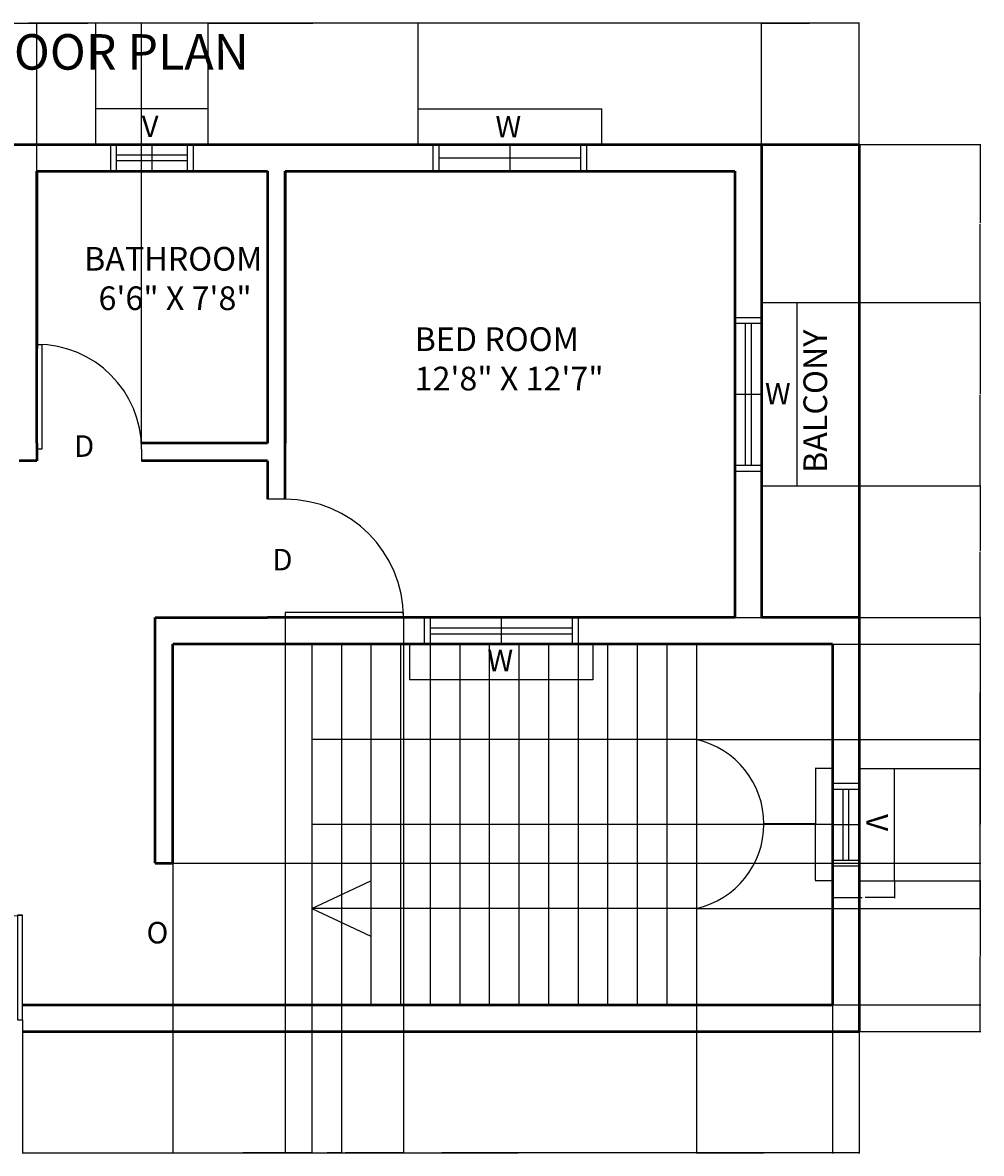
# Model space of a CAD drawing. Units: inches. Extents: x -73 to 1162, y -188 to 590.
# Tile 8 of 9: x 808 to 1132, y -187 to 195. Entities that reach past the tile are written whole.
import ezdxf

# ---------------------------------------------------------------- set-up
doc = ezdxf.new("R2010")
doc.units = ezdxf.units.IN
doc.header["$MEASUREMENT"] = 0
for name, color, linetype, lineweight in [('A-ANNO-DIMS', 2, 'Continuous', 18), ('A-ANNO-TEXT', 7, 'Continuous', 25), ('A-AREA-IDEN', 2, 'Continuous', 25), ('A-DOOR', 3, 'Continuous', 25), ('A-FLOR-STRS', 3, 'Continuous', 25), ('A-GLAZ', 4, 'Continuous', 25), ('A-WALL', 7, 'Continuous', 50)]:
    doc.layers.add(name, color=color, linetype=linetype, lineweight=lineweight)
doc.styles.get("Standard").update_dxf_attribs({"font": 'arial.ttf'})
doc.dimstyles.get("Standard").update_dxf_attribs({"dimtxt": 0.18, "dimasz": 0.18, "dimexe": 0.18, "dimexo": 0.0625, "dimgap": 0.09, "dimtad": 0, "dimtih": 1, "dimtoh": 1, "dimdec": 1, "dimzin": 0, "dimdsep": 46, "dimlunit": 4, "dimtxsty": 'Standard', "dimcen": 0.09, "dimadec": 0, "dimazin": 0, "dimtfac": 1, "dimtdec": 1, "dimtofl": 0, "dimtmove": 0, "dimatfit": 3, "dimfxl": 1, "dimtolj": 1, "dimtzin": 0, "dimarcsym": 0})

# ---------------------------------------------------------------- blocks, each defined once
blk = doc.blocks.new('*U4')
for p, q in [((0, 0), (0, -100)), ((900, 0), (900, -100))]:
    blk.add_line(p, q)
blk.add_lwpolyline([(0, 0), (0, 900), (43.75, 900), (43.75, 0)], close=True)
blk.add_arc((0, 0), 900, 0, 90)
blk = doc.blocks.new('*U7')
for p, q in [((0, 0), (0, 6)), ((40, 0), (40, 6))]:
    blk.add_line(p, q)
blk.add_lwpolyline([(0, 0), (0, -40), (1.75, -40), (1.75, 0)], close=True)
blk.add_arc((0, 0), 40, 270, 360)
blk = doc.blocks.new('WIN-W')
for p, q in [((9, 57), (9, 62)), ((9, 62), (21, 62)), ((21, 62), (21, 0)), ((0, 57), (9, 57)), ((0, 5), (9, 5)), ((9, 5), (9, 0)), ((9, 0), (21, 0))]:
    blk.add_line(p, q)
blk = doc.blocks.new('VENT-V')
for p, q in [((0, 9), (0, 21)), ((38, 21), (0, 21)), ((38, 9), (38, 21)), ((5, 9), (0, 9)), ((5, 0), (5, 9)), ((33, 0), (33, 9)), ((33, 9), (38, 9))]:
    blk.add_line(p, q)
blk = doc.blocks.new('*D32')
at = {"layer": 'A-ANNO-DIMS', "color": 0, "lineweight": -2, "transparency": 16777216}
for p, q in [((1081.24, -56.91), (1075.43, -56.91)), ((1075.61, -57.09), (1075.61, -75.72)), ((1075.61, -94.73), (1075.61, -76.09)), ((1081.24, -94.91), (1075.43, -94.91))]:
    blk.add_line(p, q, dxfattribs=at)
at = {"layer": 'A-ANNO-DIMS', "color": 0, "transparency": 16777216}
for points in [[(1075.58, -57.09), (1075.64, -57.09), (1075.61, -56.91)], [(1075.58, -94.73), (1075.64, -94.73), (1075.61, -94.91)]]:
    blk.add_solid(points, dxfattribs=at)
at = {"layer": 'Defpoints', "color": 0, "transparency": 16777216}
for p in [(1081.31, -56.91), (1075.61, -94.91), (1081.31, -94.91)]:
    blk.add_point(p, dxfattribs=at)
at = {"layer": 'A-ANNO-DIMS', "color": 0, "transparency": 16777216, "insert": (1075.61, -75.91), "char_height": 0.18, "attachment_point": 5}
blk.add_mtext('\\A1;VENTILATOR V 38 TYP.', dxfattribs=at)
blk = doc.blocks.new('*D33')
at = {"layer": 'A-ANNO-DIMS', "color": 0, "lineweight": -2, "transparency": 16777216}
for p, q in [((1081.31, -94.97), (1081.31, -100.79)), ((1102.31, -94.97), (1102.31, -100.79)), ((1081.49, -100.61), (1091.28, -100.61)), ((1102.13, -100.61), (1092.34, -100.61))]:
    blk.add_line(p, q, dxfattribs=at)
at = {"layer": 'A-ANNO-DIMS', "color": 0, "transparency": 16777216}
for points in [[(1081.49, -100.58), (1081.49, -100.64), (1081.31, -100.61)], [(1102.13, -100.58), (1102.13, -100.64), (1102.31, -100.61)]]:
    blk.add_solid(points, dxfattribs=at)
at = {"layer": 'Defpoints', "color": 0, "transparency": 16777216}
for p in [(1081.31, -94.91), (1102.31, -94.91), (1102.31, -100.61)]:
    blk.add_point(p, dxfattribs=at)
at = {"layer": 'A-ANNO-DIMS', "color": 0, "transparency": 16777216, "insert": (1091.81, -100.61), "char_height": 0.18, "attachment_point": 5}
blk.add_mtext('\\A1;21 TYP.', dxfattribs=at)
blk = doc.blocks.new('*D100')
at = {"layer": 'A-ANNO-DIMS', "color": 0, "lineweight": -2, "transparency": 16777216}
for p, q in [((557.31, 154.15), (557.31, 195.27)), ((557.49, 195.09), (823.52, 195.09)), ((1090.13, 195.09), (824.1, 195.09)), ((1090.31, 154.15), (1090.31, 195.27))]:
    blk.add_line(p, q, dxfattribs=at)
at = {"layer": 'A-ANNO-DIMS', "color": 0, "transparency": 16777216}
for points in [[(557.49, 195.12), (557.49, 195.06), (557.31, 195.09)], [(1090.13, 195.12), (1090.13, 195.06), (1090.31, 195.09)]]:
    blk.add_solid(points, dxfattribs=at)
at = {"layer": 'Defpoints', "color": 0, "transparency": 16777216}
for p in [(1090.31, 195.09), (557.31, 154.09), (1090.31, 154.09)]:
    blk.add_point(p, dxfattribs=at)
at = {"layer": 'A-ANNO-DIMS', "color": 0, "transparency": 16777216, "insert": (823.81, 195.09), "char_height": 0.18, "attachment_point": 5}
blk.add_mtext('\\A1;533', dxfattribs=at)
blk = doc.blocks.new('*D102')
at = {"layer": 'A-ANNO-DIMS', "color": 0, "lineweight": -2, "transparency": 16777216}
for p, q in [((786.31, 166.15), (786.31, 195.27)), ((786.49, 195.09), (809.08, 195.09)), ((832.13, 195.09), (809.53, 195.09)), ((832.31, 166.15), (832.31, 195.27))]:
    blk.add_line(p, q, dxfattribs=at)
at = {"layer": 'A-ANNO-DIMS', "color": 0, "transparency": 16777216}
for points in [[(786.49, 195.12), (786.49, 195.06), (786.31, 195.09)], [(832.13, 195.12), (832.13, 195.06), (832.31, 195.09)]]:
    blk.add_solid(points, dxfattribs=at)
at = {"layer": 'Defpoints', "color": 0, "transparency": 16777216}
for p in [(832.31, 195.09), (786.31, 166.09), (832.31, 166.09)]:
    blk.add_point(p, dxfattribs=at)
at = {"layer": 'A-ANNO-DIMS', "color": 0, "transparency": 16777216, "insert": (809.31, 195.09), "char_height": 0.18, "attachment_point": 5}
blk.add_mtext('\\A1;46', dxfattribs=at)
blk = doc.blocks.new('*D103')
at = {"layer": 'A-ANNO-DIMS', "color": 0, "lineweight": -2, "transparency": 16777216}
for p, q in [((870.31, 166.15), (870.31, 195.27)), ((870.49, 195.09), (905.61, 195.09)), ((941.13, 195.09), (906.01, 195.09)), ((941.31, 166.15), (941.31, 195.27))]:
    blk.add_line(p, q, dxfattribs=at)
at = {"layer": 'A-ANNO-DIMS', "color": 0, "transparency": 16777216}
for points in [[(870.49, 195.12), (870.49, 195.06), (870.31, 195.09)], [(941.13, 195.12), (941.13, 195.06), (941.31, 195.09)]]:
    blk.add_solid(points, dxfattribs=at)
at = {"layer": 'Defpoints', "color": 0, "transparency": 16777216}
for p in [(941.31, 195.09), (870.31, 166.09), (941.31, 166.09)]:
    blk.add_point(p, dxfattribs=at)
at = {"layer": 'A-ANNO-DIMS', "color": 0, "transparency": 16777216, "insert": (905.81, 195.09), "char_height": 0.18, "attachment_point": 5}
blk.add_mtext('\\A1;71', dxfattribs=at)
blk = doc.blocks.new('*D111')
at = {"layer": 'A-ANNO-DIMS', "color": 0, "lineweight": -2, "transparency": 16777216}
for p, q in [((807.52, -145.97), (807.52, -187.09)), ((1090.31, -145.97), (1090.31, -187.09)), ((807.7, -186.91), (948.52, -186.91)), ((1090.13, -186.91), (949.31, -186.91))]:
    blk.add_line(p, q, dxfattribs=at)
at = {"layer": 'A-ANNO-DIMS', "color": 0, "transparency": 16777216}
for points in [[(807.7, -186.88), (807.7, -186.94), (807.52, -186.91)], [(1090.13, -186.88), (1090.13, -186.94), (1090.31, -186.91)]]:
    blk.add_solid(points, dxfattribs=at)
at = {"layer": 'Defpoints', "color": 0, "transparency": 16777216}
for p in [(807.52, -145.91), (1090.31, -145.91), (1090.31, -186.91)]:
    blk.add_point(p, dxfattribs=at)
at = {"layer": 'A-ANNO-DIMS', "color": 0, "transparency": 16777216, "insert": (948.91, -186.91), "char_height": 0.18, "attachment_point": 5}
blk.add_mtext('\\A1;282.8', dxfattribs=at)
blk = doc.blocks.new('*D112')
at = {"layer": 'A-ANNO-DIMS', "color": 0, "lineweight": -2, "transparency": 16777216}
for p, q in [((1090.37, 154.09), (1131.49, 154.09)), ((1131.31, 153.91), (1131.31, 127.52)), ((1131.31, 100.77), (1131.31, 127.16)), ((1069.37, 100.59), (1131.49, 100.59))]:
    blk.add_line(p, q, dxfattribs=at)
at = {"layer": 'A-ANNO-DIMS', "color": 0, "transparency": 16777216}
for points in [[(1131.28, 153.91), (1131.34, 153.91), (1131.31, 154.09)], [(1131.28, 100.77), (1131.34, 100.77), (1131.31, 100.59)]]:
    blk.add_solid(points, dxfattribs=at)
at = {"layer": 'Defpoints', "color": 0, "transparency": 16777216}
for p in [(1090.31, 154.09), (1069.31, 100.59), (1131.31, 100.59)]:
    blk.add_point(p, dxfattribs=at)
at = {"layer": 'A-ANNO-DIMS', "color": 0, "transparency": 16777216, "insert": (1131.31, 127.34), "char_height": 0.18, "attachment_point": 5}
blk.add_mtext('\\A1;53.5', dxfattribs=at)
blk = doc.blocks.new('*D113')
at = {"layer": 'A-ANNO-DIMS', "color": 0, "lineweight": -2, "transparency": 16777216}
for p, q in [((1069.37, 100.59), (1131.49, 100.59)), ((1131.31, 100.41), (1131.31, 69.77)), ((1131.31, 38.77), (1131.31, 69.41)), ((1069.37, 38.59), (1131.49, 38.59))]:
    blk.add_line(p, q, dxfattribs=at)
at = {"layer": 'A-ANNO-DIMS', "color": 0, "transparency": 16777216}
for points in [[(1131.28, 100.41), (1131.34, 100.41), (1131.31, 100.59)], [(1131.28, 38.77), (1131.34, 38.77), (1131.31, 38.59)]]:
    blk.add_solid(points, dxfattribs=at)
at = {"layer": 'Defpoints', "color": 0, "transparency": 16777216}
for p in [(1069.31, 100.59), (1069.31, 38.59), (1131.31, 38.59)]:
    blk.add_point(p, dxfattribs=at)
at = {"layer": 'A-ANNO-DIMS', "color": 0, "transparency": 16777216, "insert": (1131.31, 69.59), "char_height": 0.18, "attachment_point": 5}
blk.add_mtext('\\A1;62', dxfattribs=at)
blk = doc.blocks.new('*D114')
at = {"layer": 'A-ANNO-DIMS', "color": 0, "lineweight": -2, "transparency": 16777216}
for p, q in [((1069.37, 38.59), (1131.49, 38.59)), ((1131.31, 38.41), (1131.31, 16.52)), ((1131.31, -5.73), (1131.31, 16.16)), ((1090.37, -5.91), (1131.49, -5.91))]:
    blk.add_line(p, q, dxfattribs=at)
at = {"layer": 'A-ANNO-DIMS', "color": 0, "transparency": 16777216}
for points in [[(1131.28, 38.41), (1131.34, 38.41), (1131.31, 38.59)], [(1131.28, -5.73), (1131.34, -5.73), (1131.31, -5.91)]]:
    blk.add_solid(points, dxfattribs=at)
at = {"layer": 'Defpoints', "color": 0, "transparency": 16777216}
for p in [(1069.31, 38.59), (1090.31, -5.91), (1131.31, -5.91)]:
    blk.add_point(p, dxfattribs=at)
at = {"layer": 'A-ANNO-DIMS', "color": 0, "transparency": 16777216, "insert": (1131.31, 16.34), "char_height": 0.18, "attachment_point": 5}
blk.add_mtext('\\A1;44.5', dxfattribs=at)
blk = doc.blocks.new('*D115')
at = {"layer": 'A-ANNO-DIMS', "color": 0, "lineweight": -2, "transparency": 16777216}
for p, q in [((1090.37, -5.91), (1131.49, -5.91)), ((1131.31, -6.09), (1131.31, -31.23)), ((1131.31, -56.73), (1131.31, -31.59)), ((1090.37, -56.91), (1131.49, -56.91))]:
    blk.add_line(p, q, dxfattribs=at)
at = {"layer": 'A-ANNO-DIMS', "color": 0, "transparency": 16777216}
for points in [[(1131.28, -6.09), (1131.34, -6.09), (1131.31, -5.91)], [(1131.28, -56.73), (1131.34, -56.73), (1131.31, -56.91)]]:
    blk.add_solid(points, dxfattribs=at)
at = {"layer": 'Defpoints', "color": 0, "transparency": 16777216}
for p in [(1090.31, -5.91), (1090.31, -56.91), (1131.31, -56.91)]:
    blk.add_point(p, dxfattribs=at)
at = {"layer": 'A-ANNO-DIMS', "color": 0, "transparency": 16777216, "insert": (1131.31, -31.41), "char_height": 0.18, "attachment_point": 5}
blk.add_mtext('\\A1;51', dxfattribs=at)
blk = doc.blocks.new('*D116')
at = {"layer": 'A-ANNO-DIMS', "color": 0, "lineweight": -2, "transparency": 16777216}
for p, q in [((1090.37, -94.91), (1131.49, -94.91)), ((1131.31, -95.09), (1131.31, -120.23)), ((1131.31, -145.73), (1131.31, -120.59)), ((1090.37, -145.91), (1131.49, -145.91))]:
    blk.add_line(p, q, dxfattribs=at)
at = {"layer": 'A-ANNO-DIMS', "color": 0, "transparency": 16777216}
for points in [[(1131.28, -95.09), (1131.34, -95.09), (1131.31, -94.91)], [(1131.28, -145.73), (1131.34, -145.73), (1131.31, -145.91)]]:
    blk.add_solid(points, dxfattribs=at)
at = {"layer": 'Defpoints', "color": 0, "transparency": 16777216}
for p in [(1090.31, -94.91), (1090.31, -145.91), (1131.31, -145.91)]:
    blk.add_point(p, dxfattribs=at)
at = {"layer": 'A-ANNO-DIMS', "color": 0, "transparency": 16777216, "insert": (1131.31, -120.41), "char_height": 0.18, "attachment_point": 5}
blk.add_mtext('\\A1;51', dxfattribs=at)
blk = doc.blocks.new('*D118')
at = {"layer": 'A-ANNO-DIMS', "color": 0, "lineweight": -2, "transparency": 16777216}
for p, q in [((812.31, 53.15), (812.31, 195.27)), ((812.49, 195.09), (829.6, 195.09)), ((847.5, 195.09), (830.39, 195.09)), ((847.68, 53.15), (847.68, 195.27))]:
    blk.add_line(p, q, dxfattribs=at)
at = {"layer": 'A-ANNO-DIMS', "color": 0, "transparency": 16777216}
for points in [[(812.49, 195.12), (812.49, 195.06), (812.31, 195.09)], [(847.5, 195.12), (847.5, 195.06), (847.68, 195.09)]]:
    blk.add_solid(points, dxfattribs=at)
at = {"layer": 'Defpoints', "color": 0, "transparency": 16777216}
for p in [(847.68, 195.09), (812.31, 53.09), (847.68, 53.09)]:
    blk.add_point(p, dxfattribs=at)
at = {"layer": 'A-ANNO-DIMS', "color": 0, "transparency": 16777216, "insert": (829.99, 195.09), "char_height": 0.18, "attachment_point": 5}
blk.add_mtext('\\A1;35.37', dxfattribs=at)
blk = doc.blocks.new('*D119')
at = {"layer": 'A-ANNO-DIMS', "color": 0, "lineweight": -2, "transparency": 16777216}
for p, q in [((858.31, -14.97), (858.31, -187.09)), ((905.31, -14.97), (905.31, -187.09)), ((858.49, -186.91), (881.58, -186.91)), ((905.13, -186.91), (882.03, -186.91))]:
    blk.add_line(p, q, dxfattribs=at)
at = {"layer": 'A-ANNO-DIMS', "color": 0, "transparency": 16777216}
for points in [[(858.49, -186.88), (858.49, -186.94), (858.31, -186.91)], [(905.13, -186.88), (905.13, -186.94), (905.31, -186.91)]]:
    blk.add_solid(points, dxfattribs=at)
at = {"layer": 'Defpoints', "color": 0, "transparency": 16777216}
for p in [(858.31, -14.91), (905.31, -14.91), (905.31, -186.91)]:
    blk.add_point(p, dxfattribs=at)
at = {"layer": 'A-ANNO-DIMS', "color": 0, "transparency": 16777216, "insert": (881.81, -186.91), "char_height": 0.18, "attachment_point": 5}
blk.add_mtext('\\A1;47', dxfattribs=at)
blk = doc.blocks.new('*D120')
at = {"layer": 'A-ANNO-DIMS', "color": 0, "lineweight": -2, "transparency": 16777216}
for p, q in [((905.31, -14.97), (905.31, -187.09)), ((915.31, -14.97), (915.31, -187.09)), ((905.49, -186.91), (910.1, -186.91)), ((915.13, -186.91), (910.52, -186.91))]:
    blk.add_line(p, q, dxfattribs=at)
at = {"layer": 'A-ANNO-DIMS', "color": 0, "transparency": 16777216}
for points in [[(905.49, -186.88), (905.49, -186.94), (905.31, -186.91)], [(915.13, -186.88), (915.13, -186.94), (915.31, -186.91)]]:
    blk.add_solid(points, dxfattribs=at)
at = {"layer": 'Defpoints', "color": 0, "transparency": 16777216}
for p in [(905.31, -14.91), (915.31, -14.91), (915.31, -186.91)]:
    blk.add_point(p, dxfattribs=at)
at = {"layer": 'A-ANNO-DIMS', "color": 0, "transparency": 16777216, "insert": (910.31, -186.91), "char_height": 0.18, "attachment_point": 5}
blk.add_mtext('\\A1;10', dxfattribs=at)
blk = doc.blocks.new('*D121')
at = {"layer": 'A-ANNO-DIMS', "color": 0, "lineweight": -2, "transparency": 16777216}
for p, q in [((915.31, -14.97), (915.31, -187.09)), ((1035.31, -14.97), (1035.31, -187.09)), ((915.49, -186.91), (975.03, -186.91)), ((1035.13, -186.91), (975.59, -186.91))]:
    blk.add_line(p, q, dxfattribs=at)
at = {"layer": 'A-ANNO-DIMS', "color": 0, "transparency": 16777216}
for points in [[(915.49, -186.88), (915.49, -186.94), (915.31, -186.91)], [(1035.13, -186.88), (1035.13, -186.94), (1035.31, -186.91)]]:
    blk.add_solid(points, dxfattribs=at)
at = {"layer": 'Defpoints', "color": 0, "transparency": 16777216}
for p in [(915.31, -14.91), (1035.31, -14.91), (1035.31, -186.91)]:
    blk.add_point(p, dxfattribs=at)
at = {"layer": 'A-ANNO-DIMS', "color": 0, "transparency": 16777216, "insert": (975.31, -186.91), "char_height": 0.18, "attachment_point": 5}
blk.add_mtext('\\A1;120', dxfattribs=at)
blk = doc.blocks.new('*D122')
at = {"layer": 'A-ANNO-DIMS', "color": 0, "lineweight": -2, "transparency": 16777216}
for p, q in [((1035.31, -14.97), (1035.31, -187.09)), ((1081.31, -14.97), (1081.31, -187.09)), ((1035.49, -186.91), (1058.08, -186.91)), ((1081.13, -186.91), (1058.53, -186.91))]:
    blk.add_line(p, q, dxfattribs=at)
at = {"layer": 'A-ANNO-DIMS', "color": 0, "transparency": 16777216}
for points in [[(1035.49, -186.88), (1035.49, -186.94), (1035.31, -186.91)], [(1081.13, -186.88), (1081.13, -186.94), (1081.31, -186.91)]]:
    blk.add_solid(points, dxfattribs=at)
at = {"layer": 'Defpoints', "color": 0, "transparency": 16777216}
for p in [(1035.31, -14.91), (1081.31, -14.91), (1081.31, -186.91)]:
    blk.add_point(p, dxfattribs=at)
at = {"layer": 'A-ANNO-DIMS', "color": 0, "transparency": 16777216, "insert": (1058.31, -186.91), "char_height": 0.18, "attachment_point": 5}
blk.add_mtext('\\A1;46', dxfattribs=at)
blk = doc.blocks.new('*D123')
at = {"layer": 'A-ANNO-DIMS', "color": 0, "lineweight": -2, "transparency": 16777216}
for p, q in [((852.37, -5.91), (1131.49, -5.91)), ((1131.31, -6.09), (1131.31, -47.23)), ((1131.31, -88.73), (1131.31, -47.59)), ((852.37, -88.91), (1131.49, -88.91))]:
    blk.add_line(p, q, dxfattribs=at)
at = {"layer": 'A-ANNO-DIMS', "color": 0, "transparency": 16777216}
for points in [[(1131.28, -6.09), (1131.34, -6.09), (1131.31, -5.91)], [(1131.28, -88.73), (1131.34, -88.73), (1131.31, -88.91)]]:
    blk.add_solid(points, dxfattribs=at)
at = {"layer": 'Defpoints', "color": 0, "transparency": 16777216}
for p in [(852.31, -5.91), (1131.31, -5.91), (852.31, -88.91)]:
    blk.add_point(p, dxfattribs=at)
at = {"layer": 'A-ANNO-DIMS', "color": 0, "transparency": 16777216, "insert": (1131.31, -47.41), "char_height": 0.18, "attachment_point": 5}
blk.add_mtext('\\A1;83', dxfattribs=at)
blk = doc.blocks.new('*D124')
at = {"layer": 'A-ANNO-DIMS', "color": 0, "lineweight": -2, "transparency": 16777216}
for p, q in [((1035.37, -14.91), (1131.49, -14.91)), ((1131.31, -15.09), (1131.31, -30.86)), ((1131.31, -46.99), (1131.31, -31.22)), ((1035.37, -47.17), (1131.49, -47.17))]:
    blk.add_line(p, q, dxfattribs=at)
at = {"layer": 'A-ANNO-DIMS', "color": 0, "transparency": 16777216}
for points in [[(1131.28, -15.09), (1131.34, -15.09), (1131.31, -14.91)], [(1131.28, -46.99), (1131.34, -46.99), (1131.31, -47.17)]]:
    blk.add_solid(points, dxfattribs=at)
at = {"layer": 'Defpoints', "color": 0, "transparency": 16777216}
for p in [(1035.31, -14.91), (1035.31, -47.17), (1131.31, -47.17)]:
    blk.add_point(p, dxfattribs=at)
at = {"layer": 'A-ANNO-DIMS', "color": 0, "transparency": 16777216, "insert": (1131.31, -31.04), "char_height": 0.18, "attachment_point": 5}
blk.add_mtext('\\A1;32.264', dxfattribs=at)
blk = doc.blocks.new('*D125')
at = {"layer": 'A-ANNO-DIMS', "color": 0, "lineweight": -2, "transparency": 16777216}
for p, q in [((1035.37, -47.17), (1131.49, -47.17)), ((1131.31, -47.35), (1131.31, -75.54)), ((1131.31, -104.09), (1131.31, -75.9)), ((1035.37, -104.27), (1131.49, -104.27))]:
    blk.add_line(p, q, dxfattribs=at)
at = {"layer": 'A-ANNO-DIMS', "color": 0, "transparency": 16777216}
for points in [[(1131.28, -47.35), (1131.34, -47.35), (1131.31, -47.17)], [(1131.28, -104.09), (1131.34, -104.09), (1131.31, -104.27)]]:
    blk.add_solid(points, dxfattribs=at)
at = {"layer": 'Defpoints', "color": 0, "transparency": 16777216}
for p in [(1035.31, -47.17), (1035.31, -104.27), (1131.31, -104.27)]:
    blk.add_point(p, dxfattribs=at)
at = {"layer": 'A-ANNO-DIMS', "color": 0, "transparency": 16777216, "insert": (1131.31, -75.72), "char_height": 0.18, "attachment_point": 5}
blk.add_mtext('\\A1;57.1', dxfattribs=at)
blk = doc.blocks.new('*D126')
at = {"layer": 'A-ANNO-DIMS', "color": 0, "lineweight": -2, "transparency": 16777216}
for p, q in [((1035.37, -104.27), (1131.49, -104.27)), ((1131.31, -104.45), (1131.31, -120.41)), ((1131.31, -136.73), (1131.31, -120.77)), ((1035.37, -136.91), (1131.49, -136.91))]:
    blk.add_line(p, q, dxfattribs=at)
at = {"layer": 'A-ANNO-DIMS', "color": 0, "transparency": 16777216}
for points in [[(1131.28, -104.45), (1131.34, -104.45), (1131.31, -104.27)], [(1131.28, -136.73), (1131.34, -136.73), (1131.31, -136.91)]]:
    blk.add_solid(points, dxfattribs=at)
at = {"layer": 'Defpoints', "color": 0, "transparency": 16777216}
for p in [(1035.31, -104.27), (1035.31, -136.91), (1131.31, -136.91)]:
    blk.add_point(p, dxfattribs=at)
at = {"layer": 'A-ANNO-DIMS', "color": 0, "transparency": 16777216, "insert": (1131.31, -120.59), "char_height": 0.18, "attachment_point": 5}
blk.add_mtext('\\A1;32.64', dxfattribs=at)
blk = doc.blocks.new('*D127')
at = {"layer": 'A-ANNO-DIMS', "color": 0, "lineweight": -2, "transparency": 16777216}
for p, q in [((896.31, -5.97), (896.31, -187.09)), ((936.31, -5.97), (936.31, -187.09)), ((896.49, -186.91), (916.08, -186.91)), ((936.13, -186.91), (916.53, -186.91))]:
    blk.add_line(p, q, dxfattribs=at)
at = {"layer": 'A-ANNO-DIMS', "color": 0, "transparency": 16777216}
for points in [[(896.49, -186.88), (896.49, -186.94), (896.31, -186.91)], [(936.13, -186.88), (936.13, -186.94), (936.31, -186.91)]]:
    blk.add_solid(points, dxfattribs=at)
at = {"layer": 'Defpoints', "color": 0, "transparency": 16777216}
for p in [(896.31, -5.91), (936.31, -5.91), (936.31, -186.91)]:
    blk.add_point(p, dxfattribs=at)
at = {"layer": 'A-ANNO-DIMS', "color": 0, "transparency": 16777216, "insert": (916.31, -186.91), "char_height": 0.18, "attachment_point": 5}
blk.add_mtext('\\A1;40', dxfattribs=at)
blk = doc.blocks.new('*D128')
at = {"layer": 'A-ANNO-DIMS', "color": 0, "lineweight": -2, "transparency": 16777216}
for p, q in [((1057.31, -5.85), (1057.31, 195.27)), ((1057.49, 195.09), (1073.59, 195.09)), ((1090.13, 195.09), (1074.03, 195.09)), ((1090.31, -5.85), (1090.31, 195.27))]:
    blk.add_line(p, q, dxfattribs=at)
at = {"layer": 'A-ANNO-DIMS', "color": 0, "transparency": 16777216}
for points in [[(1057.49, 195.12), (1057.49, 195.06), (1057.31, 195.09)], [(1090.13, 195.12), (1090.13, 195.06), (1090.31, 195.09)]]:
    blk.add_solid(points, dxfattribs=at)
at = {"layer": 'Defpoints', "color": 0, "transparency": 16777216}
for p in [(1090.31, 195.09), (1057.31, -5.91), (1090.31, -5.91)]:
    blk.add_point(p, dxfattribs=at)
at = {"layer": 'A-ANNO-DIMS', "color": 0, "transparency": 16777216, "insert": (1073.81, 195.09), "char_height": 0.18, "attachment_point": 5}
blk.add_mtext('\\A1;33', dxfattribs=at)
blk = doc.blocks.new('*D162')
at = {"layer": 'A-ANNO-DIMS', "color": 0, "lineweight": -2, "transparency": 16777216}
for p, q in [((1028.8, -75.72), (1028.98, -75.72)), ((1028.89, -75.81), (1028.89, -75.63)), ((1075.7, -75.69), (1058.33, -75.7))]:
    blk.add_line(p, q, dxfattribs=at)
at = {"layer": 'A-ANNO-DIMS', "color": 0, "transparency": 16777216}
blk.add_solid([(1058.33, -75.67), (1058.33, -75.73), (1058.15, -75.7)], dxfattribs=at)
at = {"layer": 'Defpoints', "color": 0, "transparency": 16777216}
for p in [(1028.89, -75.72), (1058.15, -75.7)]:
    blk.add_point(p, dxfattribs=at)
at = {"layer": 'A-ANNO-DIMS', "color": 0, "transparency": 16777216, "insert": (1076.18, -75.69), "char_height": 0.18, "attachment_point": 5}
blk.add_mtext('\\A1;R29.26', dxfattribs=at)

msp = doc.modelspace()

# ---------------------------------------------------------------- linework, layer by layer
at = {"layer": 'A-FLOR-STRS'}
for p, q in [((905.307, -14.9077), (905.307, -136.9077)), ((915.307, -14.9077), (915.307, -136.9077)), ((925.307, -14.9077), (925.307, -136.9077)), ((935.307, -14.9077), (935.307, -136.9077)), ((945.307, -14.9077), (945.307, -136.9077)), ((955.307, -14.9077), (955.307, -136.9077)), ((965.307, -14.9077), (965.307, -136.9077)), ((975.307, -14.9077), (975.307, -136.9077)), ((985.307, -14.9077), (985.307, -136.9077)), ((995.307, -14.9077), (995.307, -136.9077)), ((1005.307, -14.9077), (1005.307, -136.9077)), ((1015.307, -14.9077), (1015.307, -136.9077)), ((1025.307, -14.9077), (1025.307, -136.9077)), ((1035.307, -14.9077), (1035.307, -136.9077)), ((1035.307, -47.1714), (905.307, -47.1714)), ((1081.307, -75.9077), (905.307, -75.9077)), ((905.307, -104.2668), (925.307, -94.9497)), ((1035.307, -104.2668), (905.307, -104.2668)), ((905.307, -104.2668), (925.307, -113.5839))]:
    msp.add_line(p, q, dxfattribs=at)
msp.add_arc((1028.8864, -75.7191), 29.2608, 282.675347, 77.324653, dxfattribs=at)
at = {"layer": 'A-GLAZ'}
for p, q in [((839.307, 145.0923), (839.307, 154.0923)), ((851.307, 145.0923), (851.307, 154.0923)), ((863.307, 145.0923), (863.307, 154.0923)), ((948.307, 145.0923), (948.307, 154.0923)), ((972.307, 145.0923), (972.307, 154.0923)), ((996.307, 145.0923), (996.307, 154.0923)), ((839.307, 150.5923), (863.307, 150.5923)), ((948.307, 149.5923), (996.307, 149.5923)), ((839.307, 148.5923), (863.307, 148.5923)), ((1048.307, 93.5923), (1057.307, 93.5923)), ((1051.807, 93.5923), (1051.807, 45.5923)), ((1053.807, 93.5923), (1053.807, 45.5923)), ((1048.307, 69.5923), (1057.307, 69.5923)), ((1048.307, 45.5923), (1057.307, 45.5923)), ((943.307, -5.9077), (943.307, -14.9077)), ((945.307, -5.9077), (945.307, -14.9077)), ((969.307, -5.9077), (969.307, -14.9077)), ((993.307, -5.9077), (993.307, -14.9077)), ((995.307, -5.9077), (995.307, -14.9077)), ((945.307, -9.4077), (993.307, -9.4077)), ((945.307, -11.4077), (993.307, -11.4077)), ((943.307, -14.9077), (938.307, -14.9077)), ((938.307, -14.9077), (938.307, -26.9077)), ((995.307, -14.9077), (1000.307, -14.9077)), ((1000.307, -14.9077), (1000.307, -26.9077)), ((1000.307, -26.9077), (938.307, -26.9077)), ((1081.307, -63.9077), (1090.307, -63.9077)), ((1084.807, -63.9077), (1084.807, -87.9077)), ((1086.807, -63.9077), (1086.807, -87.9077)), ((1081.307, -75.9077), (1090.307, -75.9077)), ((1081.307, -87.9077), (1090.307, -87.9077))]:
    msp.add_line(p, q, dxfattribs=at)
at = {"layer": 'A-WALL'}
for p, q in [((728.307, 154.0923), (812.307, 154.0923)), ((812.307, 154.0923), (896.307, 154.0923)), ((896.307, 154.0923), (1090.307, 154.0923)), ((1057.307, 154.0923), (1057.307, -5.9077)), ((1090.307, 154.0923), (1090.307, -5.9077)), ((812.307, 145.0923), (812.307, 85.0923)), ((812.307, 145.0923), (890.307, 145.0923)), ((812.307, 53.0923), (812.307, 145.0923)), ((890.307, 145.0923), (890.307, 53.0923)), ((896.307, 145.0923), (896.307, 53.0923)), ((896.307, 145.0923), (1048.307, 145.0923)), ((896.307, 34.0923), (896.307, 145.0923)), ((1048.307, 145.0923), (1048.307, -5.9077)), ((812.307, 53.0923), (812.307, 47.0923)), ((890.307, 53.0923), (847.68, 53.0923)), ((812.307, 47.0923), (806.307, 47.0923)), ((890.307, 47.0923), (847.7401, 47.0923)), ((890.307, 47.0923), (890.307, 34.0923)), ((852.307, -88.9077), (852.307, -5.9077)), ((852.307, -5.9077), (890.307, -5.9077)), ((1048.307, -5.9077), (890.307, -5.9077)), ((1090.307, -5.9077), (1057.307, -5.9077)), ((1090.307, -5.9077), (1090.307, -145.9077)), ((1081.307, -14.9077), (858.307, -14.9077)), ((858.307, -88.9077), (858.307, -14.9077)), ((1081.307, -14.9077), (1081.307, -136.9077)), ((852.307, -88.9077), (858.307, -88.9077)), ((807.5207, -136.9077), (852.307, -136.9077)), ((852.307, -136.9077), (1081.307, -136.9077)), ((807.5207, -145.9077), (1090.307, -145.9077))]:
    msp.add_line(p, q, dxfattribs=at)

# ---------------------------------------------------------------- block references
at = {"layer": 'A-DOOR', "yscale": 0.0393700787401575, "zscale": 0.0393700787401575}
for p, xscale in [((812.307, 51.0293), 0.0393700787401575), ((807.5207, -141.9707), -0.0393700787401575)]:
    msp.add_blockref('*U4', p, dxfattribs=dict(at, xscale=xscale))
at = {"layer": 'A-DOOR', "rotation": 90}
msp.add_blockref('*U7', (896.307, -5.9077), dxfattribs=at)
at = {"layer": 'A-GLAZ'}
for name, p in [('VENT-V', (832.307, 145.0919)), ('WIN-W', (1048.307, 38.5919))]:
    msp.add_blockref(name, p, dxfattribs=at)
for name, p, rotation in [('WIN-W', (1003.3075, 145.0923), 90.00000000000021), ('VENT-V', (1081.3066, -56.9077), 269.999999999999)]:
    msp.add_blockref(name, p, dxfattribs=dict(at, rotation=rotation))

# ---------------------------------------------------------------- texts
at = {"layer": 'A-ANNO-TEXT'}
for s, p in [('V', (847.7724, 156.5575)), ('W', (967.3667, 156.4655)), ('W', (1058.4992, 66.1733)), ('D', (824.9009, 48.444)), ('D', (891.9441, 10.0239)), ('W', (964.6447, -24.0471)), ('O', (849.4199, -116.0969))]:
    msp.add_text(s, height=7.2829, dxfattribs=at).set_placement(p)
msp.add_text('V', height=7.2829, rotation=270, dxfattribs=at).set_placement((1092.7722, -72.3731))
at = {"layer": 'A-ANNO-TEXT', "insert": (739.1941, 191.3681), "char_height": 12, "attachment_point": 1}
msp.add_mtext_dynamic_manual_height_columns('FIRST FLOOR PLAN', width=198.609453, gutter_width=1, heights=[0], dxfattribs=at)
at = {"layer": 'A-AREA-IDEN', "char_height": 8, "attachment_point": 1}
for s, insert in [('BATHROOM\\P  6\'6" X 7\'8"', (828.2945, 119.4082)), ('BED ROOM\\P12\'8" X 12\'7"', (940.0566, 92.2393))]:
    msp.add_mtext_dynamic_manual_height_columns(s, width=71.534965, gutter_width=1, heights=[0], dxfattribs=dict(at, insert=insert))
at = {"layer": 'A-AREA-IDEN', "insert": (1071.5235, 42.9871), "char_height": 8, "attachment_point": 1, "rotation": 90}
msp.add_mtext_dynamic_manual_height_columns('BALCONY', width=71.534965, gutter_width=1, heights=[0], dxfattribs=at)

# ---------------------------------------------------------------- dimensions: what is measured, and where the dimension line sits
at = {"layer": 'A-ANNO-DIMS'}
for base, p1, p2, override, picture, middle in [((1090.307, 195.0923), (557.307, 154.0923), (1090.307, 154.0923), {"dimdec": 0, "dimlfac": 1, "dimrnd": 0, "dimzin": 0, "dimdsep": 46, "dimlunit": 2}, '*D100', (823.807, 195.0923)), ((832.307, 195.0923), (786.307, 166.0923), (832.307, 166.0923), {"dimdec": 0, "dimlfac": 1, "dimrnd": 0, "dimzin": 0, "dimdsep": 46, "dimlunit": 2}, '*D102', (809.307, 195.0923)), ((847.68, 195.0923), (812.307, 53.0923), (847.68, 53.0923), {"dimdec": 2, "dimlfac": 1, "dimrnd": 0, "dimzin": 0, "dimdsep": 46, "dimlunit": 2}, '*D118', (829.9935, 195.0923)), ((941.307, 195.0923), (870.307, 166.0923), (941.307, 166.0923), {"dimdec": 0, "dimlfac": 1, "dimrnd": 0, "dimzin": 0, "dimdsep": 46, "dimlunit": 2}, '*D103', (905.807, 195.0923)), ((1090.307, 195.0923), (1057.307, -5.9077), (1090.307, -5.9077), {"dimdec": 0, "dimlfac": 1, "dimrnd": 0, "dimzin": 0, "dimdsep": 46, "dimlunit": 2}, '*D128', (1073.807, 195.0923)), ((936.307, -186.9077), (896.307, -5.9077), (936.307, -5.9077), {"dimdec": 0, "dimlfac": 1, "dimrnd": 0, "dimzin": 0, "dimdsep": 46, "dimlunit": 2}, '*D127', (916.307, -186.9077)), ((905.307, -186.9077), (858.307, -14.9077), (905.307, -14.9077), {"dimdec": 0, "dimlfac": 1, "dimrnd": 0, "dimzin": 0, "dimdsep": 46, "dimlunit": 2}, '*D119', (881.807, -186.9077)), ((915.307, -186.9077), (905.307, -14.9077), (915.307, -14.9077), {"dimdec": 0, "dimlfac": 1, "dimrnd": 0, "dimzin": 0, "dimdsep": 46, "dimlunit": 2}, '*D120', (910.307, -186.9077)), ((1035.307, -186.9077), (915.307, -14.9077), (1035.307, -14.9077), {"dimdec": 0, "dimlfac": 1, "dimrnd": 0, "dimzin": 0, "dimdsep": 46, "dimlunit": 2}, '*D121', (975.307, -186.9077)), ((1081.307, -186.9077), (1035.307, -14.9077), (1081.307, -14.9077), {"dimdec": 0, "dimlfac": 1, "dimrnd": 0, "dimzin": 0, "dimdsep": 46, "dimlunit": 2}, '*D122', (1058.307, -186.9077)), ((1090.307, -186.9077), (807.5207, -145.9077), (1090.307, -145.9077), {"dimdec": 1, "dimlfac": 1, "dimrnd": 0, "dimzin": 0, "dimdsep": 46, "dimlunit": 2}, '*D111', (948.9139, -186.9077))]:
    dim = msp.add_linear_dim(base=base, p1=p1, p2=p2, dimstyle='Standard', override=override, dxfattribs=at)
    dim.commit()
    dim.dimension.update_dxf_attribs({"geometry": picture, "text_midpoint": middle})
for base, p1, p2, override, picture, middle in [((1131.307, 100.5923), (1090.307, 154.0923), (1069.307, 100.5923), {"dimdec": 1, "dimlfac": 1, "dimrnd": 0, "dimzin": 0, "dimdsep": 46, "dimlunit": 2}, '*D112', (1131.307, 127.3423)), ((1131.307, 38.5923), (1069.307, 100.5923), (1069.307, 38.5923), {"dimdec": 0, "dimlfac": 1, "dimrnd": 0, "dimzin": 0, "dimdsep": 46, "dimlunit": 2}, '*D113', (1131.307, 69.5923)), ((1131.307, -5.9077), (1069.307, 38.5923), (1090.307, -5.9077), {"dimdec": 1, "dimlfac": 1, "dimrnd": 0, "dimzin": 0, "dimdsep": 46, "dimlunit": 2}, '*D114', (1131.307, 16.3423)), ((1131.307, -5.9077), (852.307, -88.9077), (852.307, -5.9077), {"dimdec": 0, "dimlfac": 1, "dimrnd": 0, "dimzin": 0, "dimdsep": 46, "dimlunit": 2}, '*D123', (1131.307, -47.4077)), ((1131.307, -56.9077), (1090.307, -5.9077), (1090.307, -56.9077), {"dimdec": 0, "dimlfac": 1, "dimrnd": 0, "dimzin": 0, "dimdsep": 46, "dimlunit": 2}, '*D115', (1131.307, -31.4077)), ((1131.307, -47.1714), (1035.307, -14.9077), (1035.307, -47.1714), {"dimdec": 3, "dimlfac": 1, "dimrnd": 0, "dimzin": 0, "dimdsep": 46, "dimlunit": 2}, '*D124', (1131.307, -31.0395)), ((1131.307, -104.2668), (1035.307, -47.1714), (1035.307, -104.2668), {"dimdec": 1, "dimlfac": 1, "dimrnd": 0, "dimzin": 0, "dimdsep": 46, "dimlunit": 2}, '*D125', (1131.307, -75.7191)), ((1131.307, -145.9077), (1090.307, -94.9077), (1090.307, -145.9077), {"dimdec": 0, "dimlfac": 1, "dimrnd": 0, "dimzin": 0, "dimdsep": 46, "dimlunit": 2}, '*D116', (1131.307, -120.4077)), ((1131.307, -136.9077), (1035.307, -104.2668), (1035.307, -136.9077), {"dimdec": 2, "dimlfac": 1, "dimrnd": 0, "dimzin": 0, "dimdsep": 46, "dimlunit": 2}, '*D126', (1131.307, -120.5872))]:
    dim = msp.add_linear_dim(base=base, p1=p1, p2=p2, angle=90, dimstyle='Standard', override=override, dxfattribs=at)
    dim.commit()
    dim.dimension.update_dxf_attribs({"geometry": picture, "text_midpoint": middle})
dim = msp.add_linear_dim(base=(1075.607, -94.9077), p1=(1081.307, -56.9077), p2=(1081.307, -94.9077), angle=270, text='VENTILATOR V <> TYP.', dimstyle='Standard', override={"dimdec": 0, "dimrnd": 0, "dimzin": 0, "dimlunit": 2}, dxfattribs=at)
dim.commit()
dim.dimension.update_dxf_attribs({"geometry": '*D32', "text_midpoint": (1075.607, -75.9077)})
dim = msp.add_radius_dim(center=(1028.8864, -75.7191), mpoint=(1058.1472, -75.7), dimstyle='Standard', override={"dimdec": 2, "dimlfac": 1, "dimrnd": 0, "dimzin": 0, "dimdsep": 46, "dimlunit": 2}, dxfattribs=at)
dim.commit()
dim.dimension.update_dxf_attribs({"geometry": '*D162', "text_midpoint": (1075.7037, -75.6885), "dimtype": 164})
dim = msp.add_linear_dim(base=(1102.307, -100.6077), p1=(1081.307, -94.9077), p2=(1102.307, -94.9077), text='<> TYP.', dimstyle='Standard', override={"dimdec": 0, "dimrnd": 0, "dimzin": 0, "dimlunit": 2}, dxfattribs=at)
dim.commit()
dim.dimension.update_dxf_attribs({"geometry": '*D33', "text_midpoint": (1091.807, -100.6077)})

doc.saveas('drawing.dxf')
